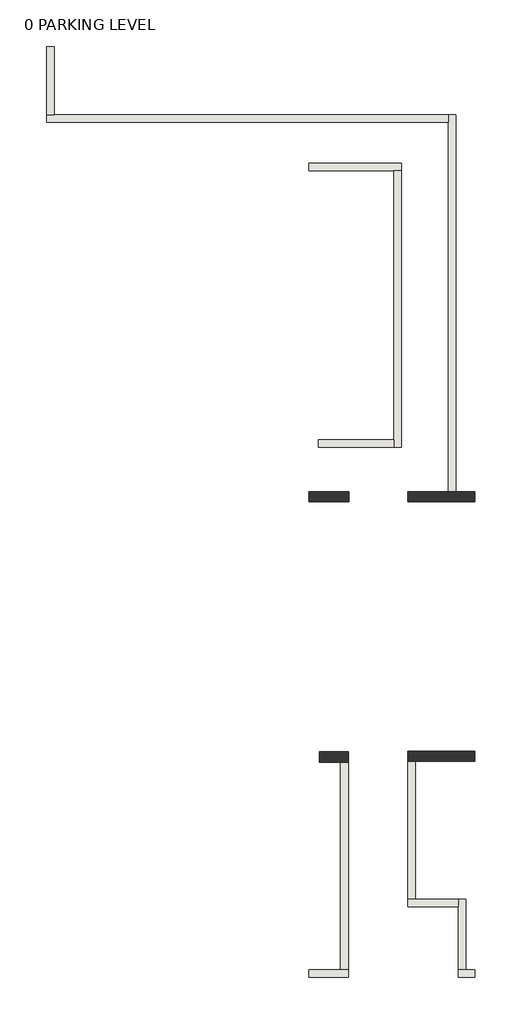
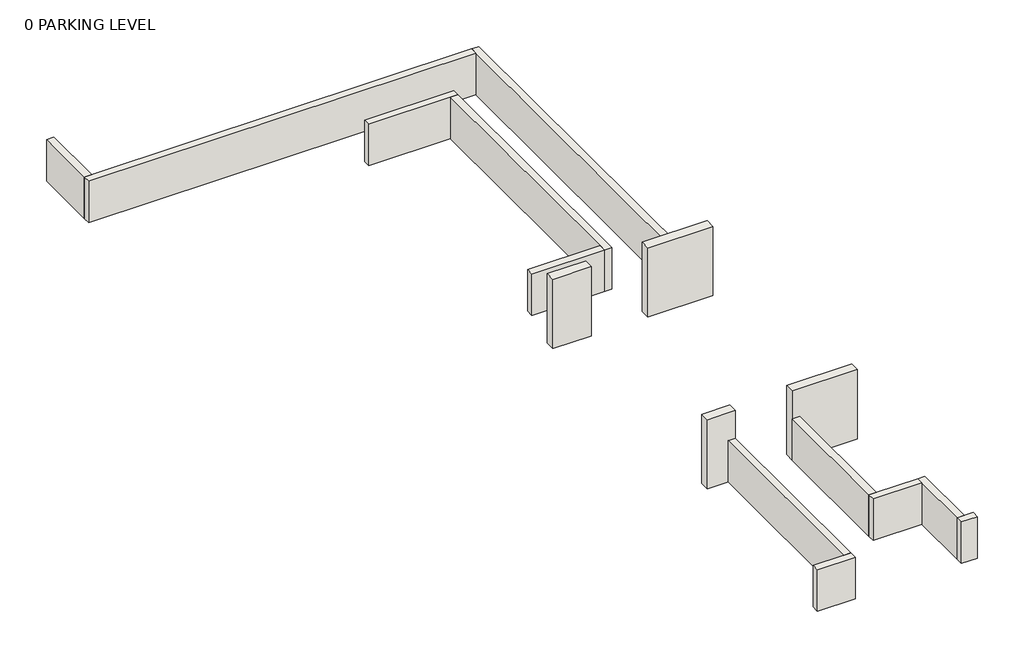
# One storey: 16 walls.
"""IFC4 building model written with IfcOpenShell, lengths in millimetres."""

from ifc_helpers import new_model, si_unit, frame, origin, place, context, project, spatial, polyline, outline, extrude, faceted_brep, element, save

model = new_model("IFC4")

# Units and contexts
model_context = context("Model", 3, world=origin())
ifc_project = project(units=[si_unit("LENGTHUNIT", "METRE", prefix="MILLI")], contexts=[model_context])

# Site, building, storey
site = spatial("IfcSite", under=ifc_project)
building = spatial("IfcBuilding", under=site)
storey = spatial("IfcBuildingStorey", under=building, Name="0 PARKING LEVEL", Elevation=-304.8)

# Walls
placement = place(None, origin())
element("IfcWall", 1, ObjectType="6", at=placement, inside=storey, context=model_context, shape_type="SweptSolid", body=[
    extrude(outline(polyline([(7972.6595608, -2470.9351307), (7972.6595608, 1700.146618), (8125.0595608, 1700.146618), (8125.0595608, -2470.9351307), (7972.6595608, -2470.9351307)])), frame((0.0, 0.0, -304.8), z_axis=(0.0, 0.0, 1.0), x_axis=(1.0, 0.0, 0.0)), (0.0, 0.0, 1.0), 914.4),
])
element("IfcWall", 2, ObjectType="6", at=placement, inside=storey, context=model_context, shape_type="Brep", body=[
    faceted_brep([(8125.0595608, -2470.9351307, -304.8), (7972.6595608, -2470.9351307, -304.8), (7338.2179176, -2470.9351307, -304.8), (7338.2179176, -2470.9351307, 609.6), (7972.6595608, -2470.9351307, 609.6), (8125.0595608, -2470.9351307, 609.6), (8125.0595608, -2623.3351307, -304.8), (8125.0595608, -2623.3351307, 609.6), (7338.2179176, -2623.3351307, 609.6), (7338.2179176, -2623.3351307, -304.8)], [[[0, 1, 2, 3, 4, 5]], [[6, 7, 8, 9]], [[2, 1, 0, 6, 9]], [[5, 4, 3, 8, 7]], [[0, 5, 7, 6]], [[3, 2, 9, 8]]]),
])
element("IfcWall", 3, ObjectType="6", at=placement, inside=storey, context=model_context, shape_type="Brep", body=[
    faceted_brep([(10672.4840945, -2470.9351307, -304.8), (10487.2595608, -2470.9351307, -304.8), (10334.8595608, -2470.9351307, -304.8), (10334.8595608, -2470.9351307, 609.6), (10487.2595608, -2470.9351307, 609.6), (10672.4840945, -2470.9351307, 609.6), (10672.4840945, -2623.3351307, -304.8), (10672.4840945, -2623.3351307, 609.6), (10334.8595608, -2623.3351307, 609.6), (10334.8595608, -2623.3351307, -304.8)], [[[0, 1, 2, 3, 4, 5]], [[6, 7, 8, 9]], [[2, 1, 0, 6, 9]], [[5, 4, 3, 8, 7]], [[3, 2, 9, 8]], [[0, 5, 7, 6]]]),
])
element("IfcWall", 4, ObjectType="6", at=placement, inside=storey, context=model_context, shape_type="Brep", body=[
    faceted_brep([(10487.2595608, -2470.9351307, -304.8), (10487.2595608, -1048.5351307, -304.8), (10487.2595608, -1048.5351307, 609.6), (10487.2595608, -2470.9351307, 609.6), (10334.8595608, -2470.9351307, -304.8), (10334.8595608, -2470.9351307, 609.6), (10334.8595608, -1200.9351307, 609.6), (10334.8595608, -1048.5351307, 609.6), (10334.8595608, -1048.5351307, -304.8), (10334.8595608, -1200.9351307, -304.8)], [[[0, 1, 2, 3]], [[4, 5, 6, 7, 8, 9]], [[1, 0, 4, 9, 8]], [[3, 2, 7, 6, 5]], [[0, 3, 5, 4]], [[2, 1, 8, 7]]]),
])
element("IfcWall", 5, ObjectType="6", at=placement, inside=storey, context=model_context, shape_type="Brep", body=[
    faceted_brep([(10334.8595608, -1048.5351307, -304.8), (9471.2595608, -1048.5351307, -304.8), (9318.8595608, -1048.5351307, -304.8), (9318.8595608, -1048.5351307, 609.6), (9471.2595608, -1048.5351307, 609.6), (10334.8595608, -1048.5351307, 609.6), (10334.8595608, -1200.9351307, -304.8), (10334.8595608, -1200.9351307, 609.6), (9318.8595608, -1200.9351307, 609.6), (9318.8595608, -1200.9351307, -304.8)], [[[0, 1, 2, 3, 4, 5]], [[6, 7, 8, 9]], [[2, 1, 0, 6, 9]], [[5, 4, 3, 8, 7]], [[0, 5, 7, 6]], [[3, 2, 9, 8]]]),
])
element("IfcWall", 6, ObjectType="6", at=placement, inside=storey, context=model_context, shape_type="SweptSolid", body=[
    extrude(outline(polyline([(9471.2595608, 1719.196618), (9471.2595608, -1048.5351307), (9318.8595608, -1048.5351307), (9318.8595608, 1719.196618), (9471.2595608, 1719.196618)])), frame((0.0, 0.0, -304.8), z_axis=(0.0, 0.0, 1.0), x_axis=(1.0, 0.0, 0.0)), (0.0, 0.0, 1.0), 914.4),
])
element("IfcWall", 7, ObjectType="6", at=placement, inside=storey, context=model_context, shape_type="Brep", body=[
    faceted_brep([(10284.0595608, 7129.396618, -304.8), (10284.0595608, 14697.0639867, -304.8), (10284.0595608, 14697.0639867, 609.6), (10284.0595608, 7129.396618, 609.6), (10131.6595608, 7129.396618, -304.8), (10131.6595608, 7129.396618, 609.6), (10131.6595608, 14544.6639867, 609.6), (10131.6595608, 14697.0639867, 609.6), (10131.6595608, 14697.0639867, -304.8), (10131.6595608, 14544.6639867, -304.8)], [[[0, 1, 2, 3]], [[4, 5, 6, 7, 8, 9]], [[1, 0, 4, 9, 8]], [[3, 2, 7, 6, 5]], [[0, 3, 5, 4]], [[2, 1, 8, 7]]]),
])
element("IfcWall", 8, ObjectType="6", at=placement, inside=storey, context=model_context, shape_type="Brep", body=[
    faceted_brep([(10131.6595608, 14697.0639867, -304.8), (2214.0821988, 14697.0639867, -304.8), (2061.6821988, 14697.0639867, -304.8), (2061.6821988, 14697.0639867, 609.6), (2214.0821988, 14697.0639867, 609.6), (10131.6595608, 14697.0639867, 609.6), (10131.6595608, 14544.6639867, -304.8), (10131.6595608, 14544.6639867, 609.6), (2061.6821988, 14544.6639867, 609.6), (2061.6821988, 14544.6639867, -304.8)], [[[0, 1, 2, 3, 4, 5]], [[6, 7, 8, 9]], [[2, 1, 0, 6, 9]], [[5, 4, 3, 8, 7]], [[0, 5, 7, 6]], [[3, 2, 9, 8]]]),
])
element("IfcWall", 9, ObjectType="6", at=placement, inside=storey, context=model_context, shape_type="SweptSolid", body=[
    extrude(outline(polyline([(2214.0821988, 16064.6306443), (2214.0821988, 14697.0639867), (2061.6821988, 14697.0639867), (2061.6821988, 16064.6306443), (2214.0821988, 16064.6306443)])), frame((0.0, 0.0, -304.8), z_axis=(0.0, 0.0, 1.0), x_axis=(1.0, 0.0, 0.0)), (0.0, 0.0, 1.0), 914.4),
])
element("IfcWall", 10, ObjectType="6", at=placement, inside=storey, context=model_context, shape_type="Brep", body=[
    faceted_brep([(7337.4638577, 13570.1893019, -304.8), (9039.4595608, 13570.1893019, -304.8), (9191.8595608, 13570.1893019, -304.8), (9191.8595608, 13570.1893019, 609.6), (9039.4595608, 13570.1893019, 609.6), (7337.4638577, 13570.1893019, 609.6), (7337.4638577, 13722.5893019, -304.8), (7337.4638577, 13722.5893019, 609.6), (9191.8595608, 13722.5893019, 609.6), (9191.8595608, 13722.5893019, -304.8)], [[[0, 1, 2, 3, 4, 5]], [[6, 7, 8, 9]], [[2, 1, 0, 6, 9]], [[5, 4, 3, 8, 7]], [[3, 2, 9, 8]], [[0, 5, 7, 6]]]),
])
element("IfcWall", 11, ObjectType="6", at=placement, inside=storey, context=model_context, shape_type="Brep", body=[
    faceted_brep([(9039.4595608, 13570.1893019, -304.8), (9039.4595608, 8170.796618, -304.8), (9039.4595608, 8018.396618, -304.8), (9039.4595608, 8018.396618, 609.6), (9039.4595608, 8170.796618, 609.6), (9039.4595608, 13570.1893019, 609.6), (9191.8595608, 13570.1893019, -304.8), (9191.8595608, 13570.1893019, 609.6), (9191.8595608, 8018.396618, 609.6), (9191.8595608, 8018.396618, -304.8)], [[[0, 1, 2, 3, 4, 5]], [[6, 7, 8, 9]], [[2, 1, 0, 6, 9]], [[5, 4, 3, 8, 7]], [[0, 5, 7, 6]], [[3, 2, 9, 8]]]),
])
element("IfcWall", 12, ObjectType="6", at=placement, inside=storey, context=model_context, shape_type="SweptSolid", body=[
    extrude(outline(polyline([(7528.1595608, 8170.796618), (9039.4595608, 8170.796618), (9039.4595608, 8018.396618), (7528.1595608, 8018.396618), (7528.1595608, 8170.796618)])), frame((0.0, 0.0, -304.8), z_axis=(0.0, 0.0, 1.0), x_axis=(1.0, 0.0, 0.0)), (0.0, 0.0, 1.0), 914.4),
])
element("IfcWall", 13, ObjectType="Generic - 8\"", at=placement, inside=storey, context=model_context, shape_type="Brep", body=[
    faceted_brep([(9318.8595608, 1719.196618, -304.8), (9471.2595608, 1719.196618, -304.8), (10672.4840945, 1719.196618, -304.8), (10672.4840945, 1719.196618, 1219.2), (9318.8595608, 1719.196618, 1219.2), (9318.8595608, 1719.196618, 609.6), (9318.8595608, 1922.396618, -304.8), (9318.8595608, 1922.396618, 1219.2), (10672.4840945, 1922.396618, 1219.2), (10672.4840945, 1922.396618, -304.8)], [[[0, 1, 2, 3, 4, 5]], [[6, 7, 8, 9]], [[2, 1, 0, 6, 9]], [[4, 3, 8, 7]], [[0, 5, 4, 7, 6]], [[3, 2, 9, 8]]]),
])
element("IfcWall", 14, ObjectType="Generic - 8\"", at=placement, inside=storey, context=model_context, shape_type="Brep", body=[
    faceted_brep([(8125.0595608, 1903.346618, -304.8), (7541.4179176, 1903.346618, -304.8), (7541.4179176, 1903.346618, 1219.2), (8125.0595608, 1903.346618, 1219.2), (8125.0595608, 1700.146618, -304.8), (8125.0595608, 1700.146618, 609.6), (8125.0595608, 1700.146618, 1219.2), (7541.4179176, 1700.146618, 1219.2), (7541.4179176, 1700.146618, -304.8), (7972.6595608, 1700.146618, -304.8)], [[[0, 1, 2, 3]], [[4, 5, 6, 7, 8, 9]], [[1, 0, 4, 9, 8]], [[3, 2, 7, 6]], [[2, 1, 8, 7]], [[0, 3, 6, 5, 4]]]),
])
element("IfcWall", 15, ObjectType="Generic - 8\"", at=placement, inside=storey, context=model_context, shape_type="SweptSolid", body=[
    extrude(outline(polyline([(7337.4638577, 7129.396618), (8137.7595608, 7129.396618), (8137.7595608, 6926.196618), (7337.4638577, 6926.196618), (7337.4638577, 7129.396618)])), frame((0.0, 0.0, -304.8), z_axis=(0.0, 0.0, 1.0), x_axis=(1.0, 0.0, 0.0)), (0.0, 0.0, 1.0), 1524.0),
])
element("IfcWall", 16, ObjectType="Generic - 8\"", at=placement, inside=storey, context=model_context, shape_type="Brep", body=[
    faceted_brep([(9318.8595608, 6926.196618, -304.8), (10672.4840945, 6926.196618, -304.8), (10672.4840945, 6926.196618, 1219.2), (9318.8595608, 6926.196618, 1219.2), (9318.8595608, 7129.396618, -304.8), (9318.8595608, 7129.396618, 1219.2), (10672.4840945, 7129.396618, 1219.2), (10672.4840945, 7129.396618, -304.8), (10284.0595608, 7129.396618, -304.8), (10131.6595608, 7129.396618, -304.8)], [[[0, 1, 2, 3]], [[4, 5, 6, 7, 8, 9]], [[1, 0, 4, 9, 8, 7]], [[3, 2, 6, 5]], [[0, 3, 5, 4]], [[2, 1, 7, 6]]]),
])

save(model, "model.ifc")

# Revit data of these elements
# Type "6"
#   Assembly Code = "B2010"
#   Layers, outside or top first: 0' - 6" no material (function 1)
# Type "Generic - 8\""
#   Assembly Code = "B2010"
#   Layers, outside or top first: 0' - 8" no material (function 1)
# Elements 1, 2, 3, 4, 5, 6, 7, 8, 9, 10, 11, 12 (IfcWall, "6")
#   Top Offset = 0' - 0"
#   Base Offset = 0' - 0"
#   Unconnected Height = 3' - 0"
#   wall height = 3' - 0"
#   Phase Created = New Construction
#   Base Constraint = 0 PARKING LEVEL
#   Materials on its faces: "Default Wall"
# Elements 13, 14, 15, 16 (IfcWall, "Generic - 8\"")
#   Top Offset = 0' - 0"
#   Base Offset = 0' - 0"
#   Unconnected Height = 5' - 0"
#   wall height = 5' - 0"
#   Phase Created = New Construction
#   Base Constraint = 0 PARKING LEVEL
#   Materials on its faces: "Default Wall"
# Materials
#   "Default Wall": colour RGB 128 128 128, transparency 0, Cost = 0
